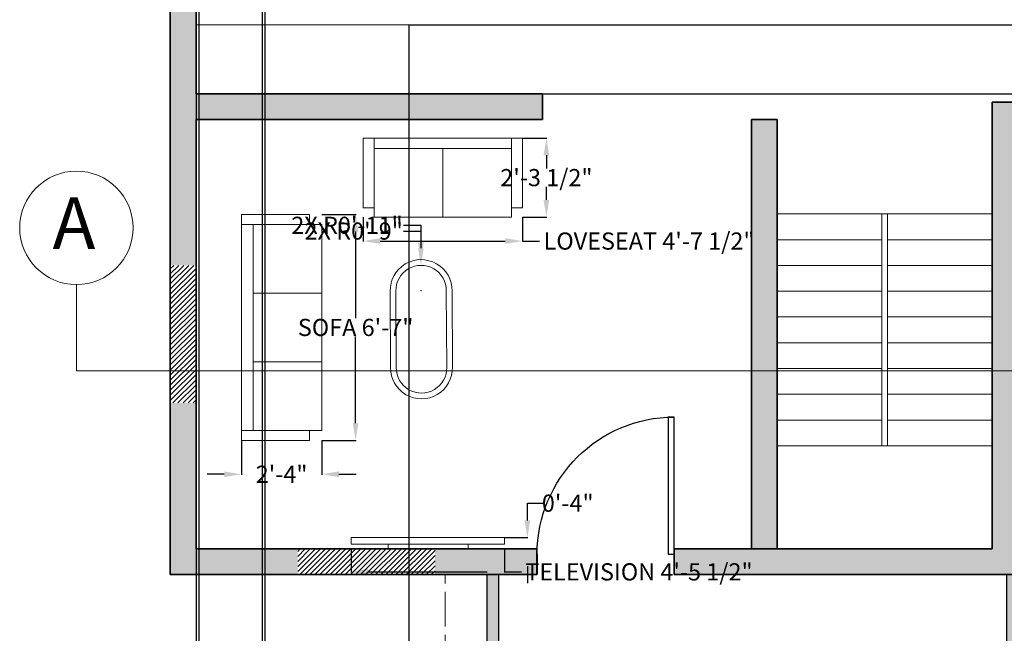
# Model space of a CAD drawing. Units: inches. Extents: x 1966 to 4198, y 2607 to 3884.
# Tile 5 of 8: x 2828 to 3172, y 3411 to 3625. Entities that reach past the tile are written whole.
import ezdxf

# ---------------------------------------------------------------- set-up
doc = ezdxf.new("R2010")
doc.units = ezdxf.units.IN
doc.header["$MEASUREMENT"] = 0
doc.linetypes.add('ACAD_ISO02W100', pattern=[15, 12, -3])
for name, color, linetype, lineweight in [('A-ANNO-SYMB', 90, 'Continuous', 18), ('A-FLOR', 7, 'Continuous', 25), ('A-FLOR-CASE', 163, 'Continuous', 18), ('A-FLOR-STRS', 7, 'Continuous', 18), ('A-GLAZ-PATT', 14, 'Continuous', 13), ('A-WALL', 7, 'Continuous', 35), ('A-WALL-PATT', 252, 'Continuous', 13), ('C-PRKG', 10, 'ACAD_ISO02W100', 18), ('dimension', 90, 'Continuous', 18), ('door', 17, 'Continuous', 25), ('furniture', 163, 'Continuous', 18)]:
    doc.layers.add(name, color=color, linetype=linetype, lineweight=lineweight)
doc.styles.get("Standard").update_dxf_attribs({"font": 'arial.ttf'})
doc.dimstyles.get("Standard").update_dxf_attribs({"dimtxt": 6, "dimasz": 6, "dimexe": 0.18, "dimexo": 0.0625, "dimgap": 0.09, "dimtad": 0, "dimtih": 1, "dimtoh": 1, "dimdec": 1, "dimzin": 0, "dimdsep": 46, "dimlunit": 3, "dimtxsty": 'Standard', "dimcen": 0.09, "dimadec": 0, "dimazin": 0, "dimtfac": 1, "dimtdec": 1, "dimtofl": 0, "dimtmove": 0, "dimatfit": 3, "dimfxl": 1, "dimtolj": 1, "dimtzin": 0, "dimarcsym": 0})

# ---------------------------------------------------------------- blocks, each defined once
blk = doc.blocks.new('S')
at = {"layer": 'furniture'}
for points in [[(2905.28, 3557.31), (2929.06, 3557.31), (2929.06, 3553.85), (2905.28, 3553.85)], [(2909.32, 3481.85), (2905.28, 3481.85), (2905.28, 3553.85), (2909.32, 3553.85)], [(2909.32, 3529.85), (2933.32, 3529.85), (2933.32, 3553.85), (2909.32, 3553.85)], [(2909.32, 3505.85), (2933.32, 3505.85), (2933.32, 3529.85), (2909.32, 3529.85)], [(2909.32, 3481.85), (2933.32, 3481.85), (2933.32, 3505.85), (2909.32, 3505.85)], [(2905.28, 3481.85), (2929.06, 3481.85), (2929.06, 3478.4), (2905.28, 3478.4)]]:
    blk.add_lwpolyline(points, close=True, dxfattribs=at)
blk = doc.blocks.new('SS')
at = {"layer": 'furniture'}
for points in [[(2953.01, 3575.89), (2956.85, 3575.89), (2956.85, 3551.48), (2953.01, 3551.48)], [(2956.85, 3572.28), (3004.85, 3572.28), (3004.85, 3575.89), (2956.85, 3575.89)], [(3004.85, 3575.89), (3008.68, 3575.89), (3008.68, 3551.48), (3004.85, 3551.48)], [(2956.85, 3548.28), (2980.85, 3548.28), (2980.85, 3572.28), (2956.85, 3572.28)], [(2980.85, 3548.28), (3004.85, 3548.28), (3004.85, 3572.28), (2980.85, 3572.28)]]:
    blk.add_lwpolyline(points, close=True, dxfattribs=at)
blk = doc.blocks.new('*U2')
for p, q in [((0, 0), (0, -6)), ((40, 0), (40, -6))]:
    blk.add_line(p, q)
blk.add_lwpolyline([(0, 0), (0, 40), (1.75, 40), (1.75, 0)], close=True)
blk.add_arc((0, 0), 40, 0, 90)
blk = doc.blocks.new('TV')
at = {"layer": 'furniture'}
for points in [[(2953.51, 3461.98), (3007.1, 3461.98), (3007.1, 3459.69), (2953.51, 3459.69)], [(2966.51, 3459.69), (2994.38, 3459.69), (2994.38, 3458.03), (2966.51, 3458.03)]]:
    blk.add_lwpolyline(points, close=True, dxfattribs=at)
blk = doc.blocks.new('STAIR-DOGLEG-PLAN')
for p, q in [((0, 81), (75, 81)), ((36.5, 0), (36.5, 81)), ((38.5, 0), (38.5, 81)), ((0, 72), (36.5, 72)), ((38.5, 72), (75, 72)), ((0, 63), (36.5, 63)), ((38.5, 63), (75, 63)), ((0, 54), (36.5, 54)), ((38.5, 54), (75, 54)), ((0, 45), (36.5, 45)), ((38.5, 45), (75, 45)), ((0, 36), (36.5, 36)), ((38.5, 36), (75, 36)), ((0, 27), (36.5, 27)), ((38.5, 27), (75, 27)), ((0, 18), (36.5, 18)), ((38.5, 18), (75, 18)), ((0, 9), (36.5, 9)), ((38.5, 9), (75, 9)), ((0, 0), (75, 0))]:
    blk.add_line(p, q)
blk = doc.blocks.new('PORCH-PARAPET-PLAN')
for p, q in [((0, 86), (0, 0)), ((4, 86), (4, 4)), ((181.42, 86), (181.42, 4)), ((185.42, 86), (185.42, 0)), ((4, 4), (23.64, 4)), ((23.64, 4), (23.64, 0)), ((83.64, 4), (83.64, 0)), ((83.64, 4), (181.42, 4)), ((0, 0), (23.64, 0)), ((83.64, 0), (185.42, 0))]:
    blk.add_line(p, q)
blk = doc.blocks.new('*D77')
at = {"layer": 'Defpoints', "color": 0, "transparency": 16777216}
for p in [(2933.32, 3557.31), (2945.16, 3557.31), (2933.32, 3478.4)]:
    blk.add_point(p, dxfattribs=at)
at = {"layer": 'dimension', "color": 0, "lineweight": -2, "transparency": 16777216}
for p, q in [((2933.38, 3557.31), (2945.34, 3557.31)), ((2945.16, 3551.31), (2945.16, 3521.05)), ((2945.16, 3484.4), (2945.16, 3514.66)), ((2933.38, 3478.4), (2945.34, 3478.4))]:
    blk.add_line(p, q, dxfattribs=at)
at = {"layer": 'dimension', "color": 0, "transparency": 16777216}
for points in [[(2944.16, 3551.31), (2946.16, 3551.31), (2945.16, 3557.31)], [(2944.16, 3484.4), (2946.16, 3484.4), (2945.16, 3478.4)]]:
    blk.add_solid(points, dxfattribs=at)
at = {"layer": 'dimension', "color": 0, "transparency": 16777216, "insert": (2945.16, 3517.85), "char_height": 6, "attachment_point": 5}
blk.add_mtext('\\A1;SOFA 6\'-7"', dxfattribs=at)
blk = doc.blocks.new('*D78')
at = {"layer": 'Defpoints', "color": 0, "transparency": 16777216}
for p in [(2905.28, 3478.4), (2933.32, 3478.4), (2933.32, 3466.56)]:
    blk.add_point(p, dxfattribs=at)
at = {"layer": 'dimension', "color": 0, "lineweight": -2, "transparency": 16777216}
for p, q in [((2905.28, 3478.33), (2905.28, 3466.38)), ((2933.32, 3478.33), (2933.32, 3466.38)), ((2899.28, 3466.56), (2893.28, 3466.56)), ((2939.32, 3466.56), (2945.32, 3466.56))]:
    blk.add_line(p, q, dxfattribs=at)
at = {"layer": 'dimension', "color": 0, "transparency": 16777216}
for points in [[(2899.28, 3467.56), (2899.28, 3465.56), (2905.28, 3466.56)], [(2939.32, 3467.56), (2939.32, 3465.56), (2933.32, 3466.56)]]:
    blk.add_solid(points, dxfattribs=at)
at = {"layer": 'dimension', "color": 0, "transparency": 16777216, "insert": (2919.3, 3466.56), "char_height": 6, "attachment_point": 5}
blk.add_mtext('\\A1;2\'-4"', dxfattribs=at)
blk = doc.blocks.new('*D79')
at = {"layer": 'Defpoints', "color": 0, "transparency": 16777216}
for p in [(2947.77, 3556.38), (3003.44, 3556.38), (3003.44, 3548.02)]:
    blk.add_point(p, dxfattribs=at)
at = {"layer": 'dimension', "color": 0, "lineweight": -2, "transparency": 16777216}
for p, q in [((2947.77, 3556.31), (2947.77, 3547.84)), ((3003.44, 3556.31), (3003.44, 3547.84)), ((2953.77, 3548.02), (2997.44, 3548.02)), ((3003.44, 3548.02), (3009.44, 3548.02))]:
    blk.add_line(p, q, dxfattribs=at)
at = {"layer": 'dimension', "color": 0, "transparency": 16777216}
for points in [[(2953.77, 3549.02), (2953.77, 3547.02), (2947.77, 3548.02)], [(2997.44, 3549.02), (2997.44, 3547.02), (3003.44, 3548.02)]]:
    blk.add_solid(points, dxfattribs=at)
at = {"layer": 'dimension', "color": 0, "transparency": 16777216, "insert": (3047.65, 3548.02), "char_height": 6, "attachment_point": 5}
blk.add_mtext('\\A1;LOVESEAT 4\'-7 1/2"', dxfattribs=at)
blk = doc.blocks.new('*D80')
at = {"layer": 'Defpoints', "color": 0, "transparency": 16777216}
for p in [(3003.44, 3583.98), (3011.79, 3583.98), (3003.44, 3556.38)]:
    blk.add_point(p, dxfattribs=at)
at = {"layer": 'dimension', "color": 0, "lineweight": -2, "transparency": 16777216}
for p, q in [((3003.5, 3583.98), (3011.97, 3583.98)), ((3011.79, 3577.98), (3011.79, 3573.37)), ((3011.79, 3562.38), (3011.79, 3566.99)), ((3003.5, 3556.38), (3011.97, 3556.38))]:
    blk.add_line(p, q, dxfattribs=at)
at = {"layer": 'dimension', "color": 0, "transparency": 16777216}
for points in [[(3010.79, 3577.98), (3012.79, 3577.98), (3011.79, 3583.98)], [(3010.79, 3562.38), (3012.79, 3562.38), (3011.79, 3556.38)]]:
    blk.add_solid(points, dxfattribs=at)
at = {"layer": 'dimension', "color": 0, "transparency": 16777216, "insert": (3011.79, 3570.18), "char_height": 6, "attachment_point": 5}
blk.add_mtext('\\A1;2\'-3 1/2"', dxfattribs=at)
blk = doc.blocks.new('*D81')
at = {"layer": 'Defpoints', "color": 0, "transparency": 16777216}
for p in [(2943.55, 3440.5), (2997.14, 3440.5), (2997.14, 3432.47)]:
    blk.add_point(p, dxfattribs=at)
at = {"layer": 'dimension', "color": 0, "lineweight": -2, "transparency": 16777216}
for p, q in [((2943.55, 3440.44), (2943.55, 3432.29)), ((2997.14, 3440.44), (2997.14, 3432.29)), ((2949.55, 3432.47), (2991.14, 3432.47)), ((2997.14, 3432.47), (3003.14, 3432.47))]:
    blk.add_line(p, q, dxfattribs=at)
at = {"layer": 'dimension', "color": 0, "transparency": 16777216}
for points in [[(2949.55, 3433.47), (2949.55, 3431.47), (2943.55, 3432.47)], [(2991.14, 3433.47), (2991.14, 3431.47), (2997.14, 3432.47)]]:
    blk.add_solid(points, dxfattribs=at)
at = {"layer": 'dimension', "color": 0, "transparency": 16777216, "insert": (3044.12, 3432.47), "char_height": 6, "attachment_point": 5}
blk.add_mtext('\\A1;TELEVISION 4\'-5 1/2"', dxfattribs=at)
blk = doc.blocks.new('*D82')
at = {"layer": 'Defpoints', "color": 0, "transparency": 16777216}
for p in [(2997.14, 3444.46), (3005.17, 3444.46), (2997.14, 3440.5)]:
    blk.add_point(p, dxfattribs=at)
at = {"layer": 'dimension', "color": 0, "lineweight": -2, "transparency": 16777216}
for p, q in [((3005.17, 3450.46), (3005.17, 3456.46)), ((3005.17, 3456.46), (3011.17, 3456.46)), ((2997.2, 3444.46), (3005.35, 3444.46)), ((2997.2, 3440.5), (3005.35, 3440.5)), ((3005.17, 3434.5), (3005.17, 3428.5))]:
    blk.add_line(p, q, dxfattribs=at)
at = {"layer": 'dimension', "color": 0, "transparency": 16777216}
for points in [[(3004.17, 3450.46), (3006.17, 3450.46), (3005.17, 3444.46)], [(3004.17, 3434.5), (3006.17, 3434.5), (3005.17, 3440.5)]]:
    blk.add_solid(points, dxfattribs=at)
at = {"layer": 'dimension', "color": 0, "transparency": 16777216, "insert": (3019.24, 3456.46), "char_height": 6, "attachment_point": 5}
blk.add_mtext('\\A1;0\'-4"', dxfattribs=at)
blk = doc.blocks.new('*D88')
at = {"layer": 'Defpoints', "color": 0, "transparency": 16777216}
for p in [(3058.44, 3836.5), (3345.44, 3203.44), (3438.28, 3203.44)]:
    blk.add_point(p, dxfattribs=at)
at = {"layer": 'dimension', "color": 0, "lineweight": -2, "transparency": 16777216}
for p, q in [((3058.5, 3836.5), (3438.46, 3836.5)), ((3438.28, 3830.5), (3438.28, 3523.13)), ((3438.28, 3209.44), (3438.28, 3516.82)), ((3345.5, 3203.44), (3438.46, 3203.44))]:
    blk.add_line(p, q, dxfattribs=at)
at = {"layer": 'dimension', "color": 0, "transparency": 16777216}
for points in [[(3437.28, 3830.5), (3439.28, 3830.5), (3438.28, 3836.5)], [(3437.28, 3209.44), (3439.28, 3209.44), (3438.28, 3203.44)]]:
    blk.add_solid(points, dxfattribs=at)
at = {"layer": 'dimension', "color": 0, "transparency": 16777216, "insert": (3438.28, 3519.97), "char_height": 6, "attachment_point": 5}
blk.add_mtext('\\A1;52\'-9"', dxfattribs=at)
blk = doc.blocks.new('*D90')
at = {"layer": 'Defpoints', "color": 0, "transparency": 16777216}
for p in [(2889.440566, 3668.990639), (2913.440566, 3668.990639), (2913.440566, 3160.931053)]:
    blk.add_point(p, dxfattribs=at)
at = {"layer": 'dimension', "color": 0, "lineweight": -2, "transparency": 16777216}
for p, q in [((2889.440566, 3668.928139), (2889.440566, 3160.751053)), ((2913.440566, 3668.928139), (2913.440566, 3160.751053)), ((2883.440566, 3160.931053), (2877.440566, 3160.931053)), ((2919.440566, 3160.931053), (2925.440566, 3160.931053))]:
    blk.add_line(p, q, dxfattribs=at)
at = {"layer": 'dimension', "color": 0, "transparency": 16777216}
for points in [[(2883.440566, 3161.931053), (2883.440566, 3159.931053), (2889.440566, 3160.931053)], [(2919.440566, 3161.931053), (2919.440566, 3159.931053), (2913.440566, 3160.931053)]]:
    blk.add_solid(points, dxfattribs=at)
at = {"layer": 'dimension', "color": 0, "transparency": 16777216, "insert": (2901.440566, 3160.931053), "char_height": 6, "attachment_point": 5}
blk.add_mtext('\\A1;2\'-0"', dxfattribs=at)
blk = doc.blocks.new('*D92')
at = {"layer": 'Defpoints', "color": 0, "transparency": 16777216}
for p in [(2889.44, 3623.5), (2963.74, 3623.5), (2963.74, 3160.93)]:
    blk.add_point(p, dxfattribs=at)
at = {"layer": 'dimension', "color": 0, "lineweight": -2, "transparency": 16777216}
for p, q in [((2889.44, 3623.44), (2889.44, 3160.75)), ((2963.74, 3623.44), (2963.74, 3160.75)), ((2895.44, 3160.93), (2911.52, 3160.93)), ((2957.74, 3160.93), (2941.66, 3160.93))]:
    blk.add_line(p, q, dxfattribs=at)
at = {"layer": 'dimension', "color": 0, "transparency": 16777216}
for points in [[(2895.44, 3161.93), (2895.44, 3159.93), (2889.44, 3160.93)], [(2957.74, 3161.93), (2957.74, 3159.93), (2963.74, 3160.93)]]:
    blk.add_solid(points, dxfattribs=at)
at = {"layer": 'dimension', "color": 0, "transparency": 16777216, "insert": (2926.59, 3160.93), "char_height": 6, "attachment_point": 5}
blk.add_mtext('\\A1;6\'-2 1/2"', dxfattribs=at)
blk = doc.blocks.new('*D93')
at = {"layer": 'Defpoints', "color": 0, "transparency": 16777216}
for p in [(2963.74, 3623.5), (3438.28, 3623.5), (2963.74, 3599.5)]:
    blk.add_point(p, dxfattribs=at)
at = {"layer": 'dimension', "color": 0, "lineweight": -2, "transparency": 16777216}
for p, q in [((2963.8, 3623.5), (3438.46, 3623.5)), ((3438.28, 3617.5), (3438.28, 3614.66)), ((3438.28, 3605.5), (3438.28, 3608.35)), ((2963.8, 3599.5), (3438.46, 3599.5))]:
    blk.add_line(p, q, dxfattribs=at)
at = {"layer": 'dimension', "color": 0, "transparency": 16777216}
for points in [[(3437.28, 3617.5), (3439.28, 3617.5), (3438.28, 3623.5)], [(3437.28, 3605.5), (3439.28, 3605.5), (3438.28, 3599.5)]]:
    blk.add_solid(points, dxfattribs=at)
at = {"layer": 'dimension', "color": 0, "transparency": 16777216, "insert": (3438.28, 3611.5), "char_height": 6, "attachment_point": 5}
blk.add_mtext('\\A1;2\'-0"', dxfattribs=at)
blk = doc.blocks.new('*D97')
at = {"layer": 'Defpoints', "color": 0, "transparency": 16777216}
for p in [(2890.43, 3707.11), (2912.55, 3707.11), (2912.55, 3160.93)]:
    blk.add_point(p, dxfattribs=at)
at = {"layer": 'dimension', "color": 0, "lineweight": -2, "transparency": 16777216}
for p, q in [((2890.43, 3707.05), (2890.43, 3160.75)), ((2912.55, 3707.05), (2912.55, 3160.75)), ((2884.43, 3160.93), (2878.43, 3160.93)), ((2918.55, 3160.93), (2924.55, 3160.93))]:
    blk.add_line(p, q, dxfattribs=at)
at = {"layer": 'dimension', "color": 0, "transparency": 16777216}
for points in [[(2884.43, 3161.93), (2884.43, 3159.93), (2890.43, 3160.93)], [(2918.55, 3161.93), (2918.55, 3159.93), (2912.55, 3160.93)]]:
    blk.add_solid(points, dxfattribs=at)
at = {"layer": 'dimension', "color": 0, "transparency": 16777216, "insert": (2901.49, 3160.93), "char_height": 6, "attachment_point": 5}
blk.add_mtext('\\A1;1\'-10"', dxfattribs=at)
blk = doc.blocks.new('*D120')
at = {"layer": 'Defpoints', "color": 0, "transparency": 16777216}
for p in [(2967.97, 3541.52), (2968.03, 3530.71)]:
    blk.add_point(p, dxfattribs=at)
at = {"layer": 'dimension', "color": 0, "lineweight": -2, "transparency": 16777216}
for p, q in [((2961.9, 3553.52), (2967.9, 3553.52)), ((2967.9, 3553.52), (2967.94, 3547.52)), ((2967.94, 3530.71), (2968.12, 3530.71)), ((2968.03, 3530.62), (2968.03, 3530.8))]:
    blk.add_line(p, q, dxfattribs=at)
at = {"layer": 'dimension', "color": 0, "transparency": 16777216}
blk.add_solid([(2968.94, 3547.52), (2966.94, 3547.51), (2967.97, 3541.52)], dxfattribs=at)
at = {"layer": 'dimension', "color": 0, "transparency": 16777216, "insert": (2942.14, 3553.52), "char_height": 6, "attachment_point": 5}
blk.add_mtext('\\A1;2X R0\'-11"', dxfattribs=at)
blk = doc.blocks.new('*D121')
at = {"layer": 'Defpoints', "color": 0, "transparency": 16777216}
for p in [(2967.98, 3539.52), (2968.03, 3530.71)]:
    blk.add_point(p, dxfattribs=at)
at = {"layer": 'dimension', "color": 0, "lineweight": -2, "transparency": 16777216}
for p, q in [((2961.91, 3551.52), (2967.91, 3551.52)), ((2967.91, 3551.52), (2967.95, 3545.52)), ((2967.94, 3530.71), (2968.12, 3530.71)), ((2968.03, 3530.62), (2968.03, 3530.8))]:
    blk.add_line(p, q, dxfattribs=at)
at = {"layer": 'dimension', "color": 0, "transparency": 16777216}
blk.add_solid([(2968.95, 3545.52), (2966.95, 3545.51), (2967.98, 3539.52)], dxfattribs=at)
at = {"layer": 'dimension', "color": 0, "transparency": 16777216, "insert": (2944.48, 3551.52), "char_height": 6, "attachment_point": 5}
blk.add_mtext('\\A1;2X R0\'-9"', dxfattribs=at)

msp = doc.modelspace()

# ---------------------------------------------------------------- hatches: boundary and pattern name
at = {"layer": 'A-GLAZ-PATT'}
h = msp.add_hatch(dxfattribs=at)
h.set_pattern_fill('ANSI31', color=256, scale=10)
h.set_pattern_definition([(45, (819.9656, 0), (-0.88388348, 0.88388348), [])])
h.paths.add_polyline_path([(2972.93, 3440.5), (2924.93, 3440.5), (2924.93, 3436), (2972.93, 3436)])
h.paths.add_polyline_path([(2972.93, 3436), (2924.93, 3436), (2924.93, 3431.5), (2972.93, 3431.5)])
h.paths.add_polyline_path([(2884.94, 3539.5), (2880.44, 3539.5), (2880.44, 3491.5), (2884.94, 3491.5)])
h.paths.add_polyline_path([(2889.44, 3539.5), (2884.94, 3539.5), (2884.94, 3491.5), (2889.44, 3491.5)])
at = {"layer": 'A-WALL-PATT'}
h = msp.add_hatch(color=256, dxfattribs=at)
h.dxf.hatch_style = 1
h.paths.add_polyline_path([(3010.44, 3599.5), (2889.44, 3599.5), (2889.44, 3698.62), (2880.44, 3698.62), (2880.44, 3590.5), (2880.44, 3539.5), (2889.44, 3539.5), (2889.44, 3590.5), (3010.44, 3590.5)])
h.paths.add_polyline_path([(2889.44, 3491.5), (2880.44, 3491.5), (2880.44, 3431.5), (2924.93, 3431.5), (2924.93, 3440.5), (2889.44, 3440.5)])
h.paths.add_polyline_path([(3008.43, 3440.5), (2972.93, 3440.5), (2972.93, 3431.5), (3008.43, 3431.5)])
h.paths.add_polyline_path([(2995.02, 3431.5), (2991.02, 3431.5), (2991.02, 3345.5), (3014.67, 3345.5), (3014.67, 3349.5), (2995.02, 3349.5)])
h.paths.add_polyline_path([(3232.44, 3440.5), (3176.44, 3440.5), (3176.44, 3587.5), (3183.92, 3587.5), (3183.92, 3591.41), (3183.92, 3596.5), (3167.44, 3596.5), (3167.44, 3440.5), (3092.44, 3440.5), (3092.44, 3590.5), (3083.44, 3590.5), (3083.44, 3440.5), (3056.43, 3440.5), (3056.43, 3438.68), (3056.43, 3431.5), (3092.44, 3431.5), (3232.44, 3431.5)])
h.paths.add_polyline_path([(3176.44, 3431.5), (3172.44, 3431.5), (3172.44, 3349.5), (3074.67, 3349.5), (3074.67, 3345.5), (3176.44, 3345.5)])
h.paths.add_polyline_path([(3345.44, 3490), (3336.44, 3490), (3336.44, 3440.5), (3280.44, 3440.5), (3280.44, 3431.5), (3345.44, 3431.5)])
h.paths.add_polyline_path([(3345.44, 3599.5), (3345.44, 3602.5), (3336.44, 3602.5), (3336.44, 3596.5), (3296.55, 3596.5), (3296.55, 3587.5), (3336.44, 3587.5), (3336.44, 3538), (3345.44, 3538)])
h.paths.add_polyline_path([(3264.44, 3632.5), (3336.44, 3632.5), (3336.44, 3626.5), (3345.44, 3626.5), (3345.44, 3692.5), (3336.44, 3692.5), (3336.44, 3641.5), (3219.92, 3641.5), (3219.92, 3632.5), (3258.44, 3632.5), (3258.44, 3596.5), (3219.95, 3596.5), (3219.95, 3591.41, -0.010779), (3219.92, 3589.86), (3219.92, 3587.5), (3268.55, 3587.5), (3268.55, 3591.7), (3268.55, 3596.5), (3264.44, 3596.5)])
h.paths.add_polyline_path([(3175.44, 3791.5), (3231.94, 3791.5), (3231.94, 3800.5), (3175.44, 3800.5), (3154.44, 3800.5), (3154.44, 3791.5), (3166.44, 3791.5), (3166.44, 3719.5), (3118.44, 3719.5), (3112.44, 3719.5), (3058.44, 3719.5), (3058.44, 3710.5), (3166.44, 3710.5), (3166.44, 3632.5), (3183.92, 3632.5), (3183.92, 3637.87), (3183.92, 3641.5), (3175.44, 3641.5)])
h.paths.add_polyline_path([(3345.44, 3800.5), (3279.94, 3800.5), (3279.94, 3791.5), (3336.44, 3791.5), (3336.44, 3740.5), (3345.44, 3740.5)])
h.paths.add_polyline_path([(3130.44, 3800.5), (3100.44, 3800.5), (3100.44, 3791.5), (3112.44, 3791.5), (3112.44, 3755.5), (3112.44, 3751.71), (3112.44, 3747.5), (3118.44, 3747.5), (3118.44, 3791.5), (3130.44, 3791.5)], flags=17)
h.paths.add_polyline_path([(3076.44, 3800.5), (3058.44, 3800.5), (3058.44, 3796.92), (3058.44, 3791.5), (3058.44, 3749.5), (3084.38, 3749.5), (3084.38, 3751.71, -0.016709), (3084.44, 3753.59), (3084.44, 3755.5), (3064.44, 3755.5), (3064.44, 3791.5), (3076.44, 3791.5)], flags=17)
h.paths.add_polyline_path([(3022.36, 3796.92, -0.017138), (3022.44, 3799.39), (3022.44, 3800.5), (3010.44, 3800.5), (2969.44, 3800.5), (2969.44, 3791.5), (3001.44, 3791.5), (3001.44, 3632.5), (3010.44, 3632.5), (3010.44, 3791.5), (3022.36, 3791.5)])
h.paths.add_polyline_path([(2921.44, 3800.5), (2880.44, 3800.5), (2880.44, 3746.62), (2889.44, 3746.62), (2889.44, 3791.5), (2921.44, 3791.5)])

# ---------------------------------------------------------------- linework, layer by layer
at = {"layer": 'A-ANNO-SYMB'}
for p, q in [((2847.64, 3532.82), (2847.64, 3502.67)), ((2847.64, 3502.67), (3380.97, 3502.67))]:
    msp.add_line(p, q, dxfattribs=at)
msp.add_circle((2847.64, 3552.63), 19.81, dxfattribs=at)
at = {"layer": 'A-FLOR-CASE'}
for p, q in [((2889.44, 3623.5), (2963.74, 3623.5)), ((2963.74, 3623.5), (2963.74, 3599.5))]:
    msp.add_line(p, q, dxfattribs=at)
at = {"layer": 'A-WALL'}
for p, q in [((2880.44, 3800.5), (2880.44, 3590.5)), ((2889.44, 3791.5), (2889.44, 3599.5)), ((2889.44, 3599.5), (3010.44, 3599.5)), ((3010.44, 3590.5), (3010.44, 3599.5)), ((3167.44, 3596.5), (3183.92, 3596.5)), ((3167.44, 3440.5), (3167.44, 3596.5)), ((2880.44, 3431.5), (2880.44, 3590.5)), ((2889.44, 3590.5), (3010.44, 3590.5)), ((2889.44, 3440.5), (2889.44, 3590.5)), ((3083.44, 3440.5), (3083.44, 3590.5)), ((3083.44, 3590.5), (3092.44, 3590.5)), ((3092.44, 3440.5), (3092.44, 3590.5)), ((2889.44, 3440.5), (3008.43, 3440.5)), ((3008.43, 3440.5), (3008.43, 3431.5)), ((3056.43, 3440.5), (3083.44, 3440.5)), ((3056.43, 3440.5), (3056.43, 3431.5)), ((3083.44, 3440.5), (3092.44, 3440.5)), ((3092.44, 3440.5), (3167.44, 3440.5)), ((2880.44, 3431.5), (3008.43, 3431.5)), ((3056.43, 3431.5), (3092.44, 3431.5)), ((3092.44, 3431.5), (3345.44, 3431.5))]:
    msp.add_line(p, q, dxfattribs=at)
at = {"layer": 'C-PRKG'}
msp.add_line((2976.4, 3203.44), (2976.4, 3431.5), dxfattribs=at)
at = {"layer": 'furniture'}
for points in [[(2957.37, 3503.86), (2957.22, 3530.45)], [(2959.37, 3503.87), (2959.22, 3530.46)], [(2976.84, 3530.56), (2976.99, 3503.97)], [(2978.84, 3530.57), (2978.99, 3503.98)]]:
    msp.add_lwpolyline(points, dxfattribs=at)
for centre, radius, start, end in [((2968.03, 3530.71), 10.81, 359.2861, 181.3581), ((2968.03, 3530.71), 8.81, 359.2861, 181.3581), ((2968.18, 3503.72), 10.81, 179.2861, 1.3581), ((2968.18, 3503.72), 8.81, 179.2861, 1.3581)]:
    msp.add_arc(centre, radius, start, end, dxfattribs=at)

# ---------------------------------------------------------------- block references
at = {"layer": 'A-FLOR'}
msp.add_blockref('PORCH-PARAPET-PLAN', (2991.02, 3345.5), dxfattribs=at)
at = {"layer": 'A-FLOR-STRS'}
msp.add_blockref('STAIR-DOGLEG-PLAN', (3092.44, 3476.5), dxfattribs=at)
at = {"layer": 'door', "xscale": -1.196636277150106, "yscale": 1.196636277150106, "zscale": 1.196636277150106}
msp.add_blockref('*U2', (3056.43, 3438.68), dxfattribs=at)
at = {"layer": 'furniture'}
for name, p in [('SS', (-5.24, 8.09)), ('S', (0, 0)), ('TV', (-9.96, -17.53))]:
    msp.add_blockref(name, p, dxfattribs=at)

# ---------------------------------------------------------------- texts
at = {"layer": 'A-ANNO-SYMB', "insert": (2839.31, 3563.3), "char_height": 18, "attachment_point": 1}
msp.add_mtext_dynamic_manual_height_columns('A', width=16.3986, gutter_width=1, heights=[0], dxfattribs=at)

# ---------------------------------------------------------------- dimensions: what is measured, and where the dimension line sits
at = {"layer": 'dimension'}
for base, p1, p2, picture, middle in [((3438.28, 3203.44), (3058.44, 3836.5), (3345.44, 3203.44), '*D88', (3438.28, 3519.97)), ((3438.28, 3623.5), (2963.74, 3599.5), (2963.74, 3623.5), '*D93', (3438.28, 3611.5)), ((3011.79, 3583.98), (3003.44, 3556.38), (3003.44, 3583.98), '*D80', (3011.79, 3570.18)), ((3005.17, 3444.46), (2997.14, 3440.5), (2997.14, 3444.46), '*D82', (3019.24, 3456.46))]:
    dim = msp.add_linear_dim(base=base, p1=p1, p2=p2, angle=90, dimstyle='Standard', override={"dimdec": 1, "dimlfac": 1, "dimrnd": 0, "dimzin": 1, "dimdsep": 46, "dimlunit": 4, "dimfrac": 2}, dxfattribs=at)
    dim.commit()
    dim.dimension.update_dxf_attribs({"geometry": picture, "text_midpoint": middle})
for base, p1, p2, picture, middle in [((2912.55, 3160.93), (2890.43, 3707.11), (2912.55, 3707.11), '*D97', (2901.49, 3160.93)), ((2913.44, 3160.93), (2889.44, 3668.99), (2913.44, 3668.99), '*D90', (2901.44, 3160.93)), ((2963.74, 3160.93), (2889.44, 3623.5), (2963.74, 3623.5), '*D92', (2926.59, 3160.93)), ((2933.32, 3466.56), (2905.28, 3478.4), (2933.32, 3478.4), '*D78', (2919.3, 3466.56))]:
    dim = msp.add_linear_dim(base=base, p1=p1, p2=p2, dimstyle='Standard', override={"dimdec": 1, "dimlfac": 1, "dimrnd": 0, "dimzin": 1, "dimdsep": 46, "dimlunit": 4, "dimfrac": 2}, dxfattribs=at)
    dim.commit()
    dim.dimension.update_dxf_attribs({"geometry": picture, "text_midpoint": middle})
for mpoint, picture, middle in [((2967.97, 3541.52), '*D120', (2942.14, 3553.52)), ((2967.98, 3539.52), '*D121', (2944.48, 3551.52))]:
    dim = msp.add_radius_dim(center=(2968.03, 3530.71), mpoint=mpoint, text='2X <>', dimstyle='Standard', override={"dimdec": 1, "dimlfac": 1, "dimrnd": 0, "dimzin": 1, "dimdsep": 46, "dimlunit": 4, "dimfrac": 2}, dxfattribs=at)
    dim.commit()
    dim.dimension.update_dxf_attribs({"geometry": picture, "text_midpoint": middle})
for base, p1, p2, text, picture, middle in [((3003.44, 3548.02), (2947.77, 3556.38), (3003.44, 3556.38), 'LOVESEAT <>', '*D79', (3047.65, 3548.02)), ((2997.14, 3432.47), (2943.55, 3440.5), (2997.14, 3440.5), 'TELEVISION <>', '*D81', (3044.12, 3432.47))]:
    dim = msp.add_linear_dim(base=base, p1=p1, p2=p2, text=text, dimstyle='Standard', override={"dimdec": 1, "dimlfac": 1, "dimrnd": 0, "dimzin": 1, "dimdsep": 46, "dimlunit": 4, "dimfrac": 2}, dxfattribs=at)
    dim.commit()
    dim.dimension.update_dxf_attribs({"geometry": picture, "text_midpoint": middle})
dim = msp.add_linear_dim(base=(2945.16, 3557.31), p1=(2933.32, 3478.4), p2=(2933.32, 3557.31), angle=90, text='SOFA <>', dimstyle='Standard', override={"dimdec": 1, "dimlfac": 1, "dimrnd": 0, "dimzin": 1, "dimdsep": 46, "dimlunit": 4, "dimfrac": 2}, dxfattribs=at)
dim.commit()
dim.dimension.update_dxf_attribs({"geometry": '*D77', "text_midpoint": (2945.16, 3517.85)})

doc.saveas('drawing.dxf')
